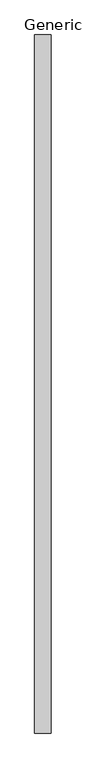
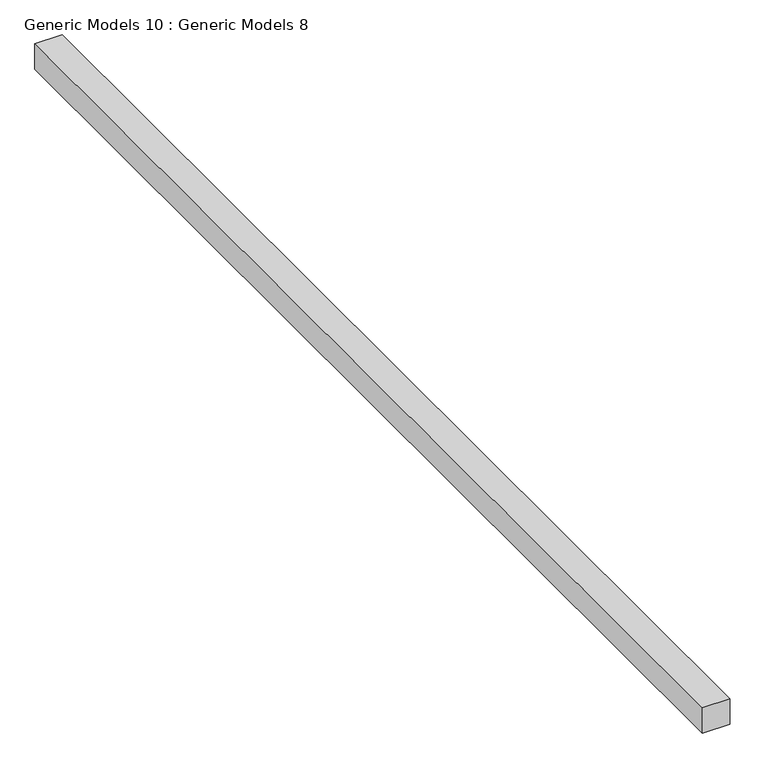
"""IFC4 building model written with IfcOpenShell, lengths in millimetres: proxy geometry, Generic Models 10 : Generic Models 8."""

from ifc_helpers import new_model, si_unit, frame, origin, place, context, project, spatial, polyline, outline, extrude, source, transform, mapped, element, save


def generic_models_10_generic_models_8_4a409525(model_context):
    return source(origin(), model_context, "Body", "SweptSolid", [
        extrude(outline(polyline([(-14138.2638778, 4522.2475408), (-14138.2638778, 17411.9959632), (-13833.4638778, 17411.9959632), (-13833.4638778, 4522.2475408), (-14138.2638778, 4522.2475408)])), frame((0.0, 0.0, 18436.4628525), z_axis=(0.0, 0.0, 1.0), x_axis=(1.0, 0.0, 0.0)), (0.0, 0.0, 1.0), 299.4321768),
    ])


if __name__ == "__main__":
    model = new_model("IFC4")
    model_context = context("Model", 3, world=origin())
    ifc_project = project(units=[si_unit("LENGTHUNIT", "METRE", prefix="MILLI")], contexts=[model_context])
    site = spatial("IfcSite", under=ifc_project)
    building = spatial("IfcBuilding", under=site)
    placement = place(None, origin())
    generic_models_10_generic_models_8_shape = generic_models_10_generic_models_8_4a409525(model_context)
    element("IfcBuildingElementProxy", 1, Name="Generic Models 10 : Generic Models 8", ObjectType="Generic Models 10 : Generic Models 8", at=placement, inside=building, context=model_context, shape_type="MappedRepresentation", body=[
        mapped(generic_models_10_generic_models_8_shape, transform((0.0, 0.0, 0.0), x_axis=(1.0, 0.0, 0.0), y_axis=(0.0, 1.0, 0.0), z_axis=(0.0, 0.0, 1.0))),
    ])
    save(model, "model.ifc")
